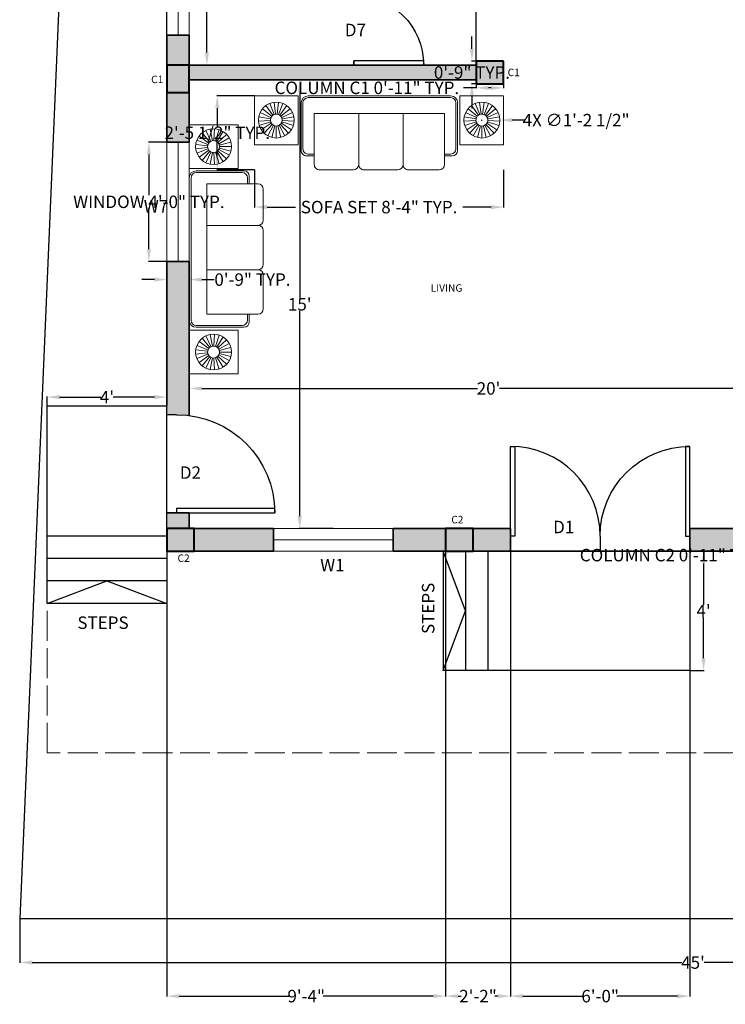
# Model space of a CAD drawing. Units: inches. Extents: x 23868 to 24454, y 31838 to 32477.
# Tile 1 of 4: x 23868 to 24151, y 31838 to 32233. Entities that reach past the tile are written whole.
import ezdxf

# ---------------------------------------------------------------- set-up
doc = ezdxf.new("R2010")
doc.units = ezdxf.units.IN
doc.linetypes.add('ACAD_ISO02W100', pattern=[15, 12, -3])
for name, color, linetype, lineweight in [('A-ANNO-DIMS', 2, 'Continuous', 18), ('A-AREA-IDEN', 7, 'Continuous', 25), ('A-COLS', 7, 'Continuous', 40), ('A-FURN', 30, 'Continuous', 18), ('A-GLAZ', 5, 'Continuous', 18), ('A-WALL', 7, 'Continuous', 35), ('C-PROP', 7, 'Continuous', 25), ('door', 1, 'Continuous', 25), ('steps', 104, 'Continuous', 25), ('text', 7, 'Continuous', 18)]:
    doc.layers.add(name, color=color, linetype=linetype, lineweight=lineweight)
for name, color, linetype, lineweight, true_color in [('A-COLS-PATT', 67, 'Continuous', 13, 0x727430), ('A-FLOR-OVHD', 244, 'ACAD_ISO02W100', 18, 0x991b1e), ('A-WALL-PATT', 250, 'Continuous', 13, 0x413a3c)]:
    doc.layers.add(name, color=color, linetype=linetype, lineweight=lineweight, true_color=true_color)
doc.styles.get("Standard").update_dxf_attribs({"font": 'arial.ttf', "height": 5})
doc.styles.add('style1', font='arial.ttf', dxfattribs={"height": 3})
doc.dimstyles.get("Standard").update_dxf_attribs({"dimtxt": 5, "dimasz": 5, "dimexe": 0.18, "dimexo": 0.0625, "dimgap": 0.09, "dimtad": 0, "dimtih": 1, "dimtoh": 1, "dimzin": 0, "dimdsep": 46, "dimlunit": 3, "dimtxsty": 'Standard', "dimcen": 0.09, "dimadec": 0, "dimazin": 0, "dimtfac": 1, "dimtofl": 0, "dimtmove": 0, "dimatfit": 3, "dimfxl": 1, "dimtolj": 1, "dimtzin": 0, "dimarcsym": 0})

# ---------------------------------------------------------------- blocks, each defined once
blk = doc.blocks.new('*U2')
for p, q in [((0, 0), (0, -100)), ((1000, 0), (1000, -100))]:
    blk.add_line(p, q)
blk.add_lwpolyline([(0, 0), (0, 1000), (43.75, 1000), (43.75, 0)], close=True)
blk.add_arc((0, 0), 1000, 0, 90)
blk = doc.blocks.new('*U6')
for p, q in [((0, 0), (0, -6)), ((36, 0), (36, -6))]:
    blk.add_line(p, q)
blk.add_lwpolyline([(0, 0), (0, 36), (1.75, 36), (1.75, 0)], close=True)
blk.add_arc((0, 0), 36, 0, 90)
blk = doc.blocks.new('*U5')
for p, q in [((0, 0), (0, -6)), ((28, 0), (28, -6))]:
    blk.add_line(p, q)
blk.add_lwpolyline([(0, 0), (0, 28), (1.75, 28), (1.75, 0)], close=True)
blk.add_arc((0, 0), 28, 0, 90)
blk = doc.blocks.new('sofa')
for p, q in [((-58.2, 3.63), (-60.24, 7.96)), ((-57.63, 3.81), (-58.53, 8.51)), ((-57.03, 3.85), (-56.73, 8.63)), ((-56.44, 3.74), (-54.97, 8.29)), ((-59.41, 2.34), (-63.86, 4.1)), ((-59.12, 2.87), (-62.99, 5.68)), ((-58.71, 3.3), (-61.76, 6.99)), ((-55.9, 3.48), (-53.34, 7.52)), ((-55.44, 3.1), (-51.95, 6.38)), ((-55.09, 2.61), (-50.89, 4.92)), ((-59.56, 1.76), (-64.31, 2.36)), ((-59.56, 1.16), (-64.31, 0.56)), ((-59.41, 0.58), (-63.86, -1.18)), ((-59.12, 0.05), (-62.99, -2.76)), ((-55.09, 0.31), (-50.89, -2)), ((-54.87, 2.06), (-50.23, 3.25)), ((-54.87, 0.86), (-50.23, -0.33)), ((-54.79, 1.46), (-50, 1.46)), ((-58.71, -0.38), (-61.76, -4.07)), ((-58.2, -0.71), (-60.24, -5.04)), ((-57.63, -0.89), (-58.53, -5.59)), ((-57.03, -0.93), (-56.73, -5.71)), ((-56.44, -0.82), (-54.97, -5.37)), ((-55.9, -0.56), (-53.34, -4.6)), ((-55.44, -0.18), (-51.95, -3.46)), ((-66.9, -68.18), (-66.9, -11.07)), ((-66.2, -68.18), (-66.2, -11.07)), ((-44.98, -8.25), (-64.08, -8.25)), ((-45.68, -8.96), (-64.08, -8.96)), ((-43.56, -13.5), (-43.56, -11.07)), ((-42.86, -13.5), (-42.86, -10.37)), ((-59.86, -13.5), (-39.37, -13.5)), ((-59.86, -65.75), (-59.86, -13.5)), ((-37.25, -15.62), (-37.25, -28.01)), ((-39.37, -30.13), (-59.86, -30.13)), ((-37.25, -32.25), (-37.25, -45.82)), ((-39.37, -47.94), (-59.86, -47.94)), ((-37.25, -50.06), (-37.25, -63.63)), ((-39.37, -65.75), (-59.86, -65.75)), ((-43.56, -65.75), (-43.56, -68.18)), ((-42.86, -65.75), (-42.86, -68.89)), ((-45.68, -70.3), (-64.08, -70.3)), ((-44.98, -71.01), (-64.08, -71.01)), ((-58.2, -78.8), (-60.24, -74.47)), ((-57.63, -78.62), (-58.53, -73.92)), ((-57.03, -78.58), (-56.73, -73.8)), ((-56.44, -78.69), (-54.97, -74.14)), ((-55.9, -78.95), (-53.34, -74.91)), ((-59.41, -80.09), (-63.86, -78.33)), ((-59.12, -79.56), (-62.99, -76.75)), ((-58.71, -79.12), (-61.76, -75.44)), ((-55.44, -79.33), (-51.95, -76.05)), ((-55.09, -79.82), (-50.89, -77.51)), ((-59.56, -80.67), (-64.31, -80.07)), ((-59.56, -81.27), (-64.31, -81.87)), ((-59.41, -81.85), (-63.86, -83.61)), ((-59.12, -82.38), (-62.99, -85.19)), ((-58.71, -82.81), (-61.76, -86.5)), ((-55.44, -82.61), (-51.95, -85.88)), ((-55.09, -82.12), (-50.89, -84.43)), ((-54.87, -80.37), (-50.23, -79.18)), ((-54.87, -81.56), (-50.23, -82.75)), ((-54.79, -80.97), (-50, -80.97)), ((-58.2, -83.13), (-60.24, -87.47)), ((-57.63, -83.32), (-58.53, -88.02)), ((-57.03, -83.36), (-56.73, -88.14)), ((-56.44, -83.25), (-54.97, -87.8)), ((-55.9, -82.99), (-53.34, -87.03))]:
    blk.add_line(p, q)
for points in [[(-66.96, 10.15), (-47.26, 10.15), (-47.26, -7.32), (-66.96, -7.32)], [(-66.96, -89.66), (-47.26, -89.66), (-47.26, -72.19), (-66.96, -72.19)]]:
    blk.add_lwpolyline(points, close=True)
for centre, radius in [((-57.18, 1.46), 7.18), ((-57.18, 1.46), 2.39), ((-57.18, -80.97), 7.18), ((-57.18, -80.97), 2.39)]:
    blk.add_circle(centre, radius)
for centre, radius, start, end in [((-64.08, -11.07), 2.83, 90, 180), ((-64.08, -11.07), 2.12, 90, 180), ((-45.68, -11.07), 2.12, 0, 90), ((-44.98, -10.37), 2.12, 0, 90), ((-39.37, -15.62), 2.12, 0, 90), ((-39.37, -28.01), 2.12, 270, 0), ((-39.37, -32.25), 2.12, 0, 90), ((-39.37, -45.82), 2.12, 270, 0), ((-39.37, -50.06), 2.12, 0, 90), ((-39.37, -63.63), 2.12, 270, 0), ((-64.08, -68.18), 2.83, 180, 270), ((-64.08, -68.18), 2.12, 180, 270), ((-45.68, -68.18), 2.12, 270, 0), ((-44.98, -68.89), 2.12, 270, 0)]:
    blk.add_arc(centre, radius, start, end)
blk = doc.blocks.new('*D30')
at = {"layer": 'A-ANNO-DIMS', "color": 0, "lineweight": -2, "transparency": 16777216}
for p, q in [((23879.1, 32077.73), (23879.1, 32081.55)), ((23884.1, 32081.37), (23900.61, 32081.37)), ((23922.1, 32081.37), (23905.59, 32081.37)), ((23927.1, 32077.73), (23927.1, 32081.55))]:
    blk.add_line(p, q, dxfattribs=at)
at = {"layer": 'A-ANNO-DIMS', "color": 0, "transparency": 16777216}
for points in [[(23884.1, 32082.2), (23884.1, 32080.54), (23879.1, 32081.37)], [(23922.1, 32082.2), (23922.1, 32080.54), (23927.1, 32081.37)]]:
    blk.add_solid(points, dxfattribs=at)
at = {"layer": 'Defpoints', "color": 0, "transparency": 16777216}
for p in [(23879.1, 32081.37), (23879.1, 32077.66), (23927.1, 32077.66)]:
    blk.add_point(p, dxfattribs=at)
at = {"layer": 'A-ANNO-DIMS', "color": 0, "transparency": 16777216, "insert": (23903.1, 32081.37), "char_height": 5, "attachment_point": 5}
blk.add_mtext("\\A1;4'", dxfattribs=at)
blk = doc.blocks.new('*D33')
at = {"layer": 'A-ANNO-DIMS', "color": 0, "lineweight": -2, "transparency": 16777216}
for p, q in [((23936.1, 32084.78), (23936.1, 32084.66)), ((23941.1, 32084.84), (24051.72, 32084.84)), ((24171.1, 32084.84), (24060.48, 32084.84)), ((24176.1, 32084.9), (24176.1, 32085.02))]:
    blk.add_line(p, q, dxfattribs=at)
at = {"layer": 'A-ANNO-DIMS', "color": 0, "transparency": 16777216}
for points in [[(23941.1, 32085.67), (23941.1, 32084.01), (23936.1, 32084.84)], [(24171.1, 32085.67), (24171.1, 32084.01), (24176.1, 32084.84)]]:
    blk.add_solid(points, dxfattribs=at)
at = {"layer": 'Defpoints', "color": 0, "transparency": 16777216}
for p in [(23936.1, 32084.84), (24176.1, 32084.84), (24176.1, 32084.84)]:
    blk.add_point(p, dxfattribs=at)
at = {"layer": 'A-ANNO-DIMS', "color": 0, "transparency": 16777216, "insert": (24056.1, 32084.84), "char_height": 5, "attachment_point": 5}
blk.add_mtext("\\A1;20'", dxfattribs=at)
blk = doc.blocks.new('*D34')
at = {"layer": 'A-ANNO-DIMS', "color": 0, "lineweight": -2, "transparency": 16777216}
for p, q in [((23993.53, 32208.61), (23980.21, 32208.61)), ((23980.39, 32203.61), (23980.39, 32121.25)), ((23980.39, 32033.61), (23980.39, 32115.97)), ((23993.76, 32028.61), (23980.21, 32028.61))]:
    blk.add_line(p, q, dxfattribs=at)
at = {"layer": 'A-ANNO-DIMS', "color": 0, "transparency": 16777216}
for points in [[(23979.56, 32203.61), (23981.22, 32203.61), (23980.39, 32208.61)], [(23979.56, 32033.61), (23981.22, 32033.61), (23980.39, 32028.61)]]:
    blk.add_solid(points, dxfattribs=at)
at = {"layer": 'Defpoints', "color": 0, "transparency": 16777216}
for p in [(23980.39, 32208.61), (23993.59, 32208.61), (23993.83, 32028.61)]:
    blk.add_point(p, dxfattribs=at)
at = {"layer": 'A-ANNO-DIMS', "color": 0, "transparency": 16777216, "insert": (23980.39, 32118.61), "char_height": 5, "attachment_point": 5}
blk.add_mtext("\\A1;15'", dxfattribs=at)
blk = doc.blocks.new('*D35')
at = {"layer": 'A-ANNO-DIMS', "color": 0, "lineweight": -2, "transparency": 16777216}
for p, q in [((23936.16, 32262.61), (23943.36, 32262.61)), ((23943.18, 32257.61), (23943.18, 32241.2)), ((23943.18, 32219.61), (23943.18, 32236.02)), ((23936.16, 32214.61), (23943.36, 32214.61))]:
    blk.add_line(p, q, dxfattribs=at)
at = {"layer": 'A-ANNO-DIMS', "color": 0, "transparency": 16777216}
for points in [[(23942.35, 32257.61), (23944.01, 32257.61), (23943.18, 32262.61)], [(23942.35, 32219.61), (23944.01, 32219.61), (23943.18, 32214.61)]]:
    blk.add_solid(points, dxfattribs=at)
at = {"layer": 'Defpoints', "color": 0, "transparency": 16777216}
for p in [(23936.1, 32262.61), (23943.18, 32262.61), (23936.1, 32214.61)]:
    blk.add_point(p, dxfattribs=at)
at = {"layer": 'A-ANNO-DIMS', "color": 0, "transparency": 16777216, "insert": (23943.18, 32238.61), "char_height": 5, "attachment_point": 5}
blk.add_mtext("\\A1;4'", dxfattribs=at)
blk = doc.blocks.new('*D39')
at = {"layer": 'A-ANNO-DIMS', "color": 0, "lineweight": -2, "transparency": 16777216}
for p, q in [((24136.92, 32019.61), (24142.52, 32019.61)), ((24142.34, 32014.61), (24142.34, 31998.2)), ((24142.34, 31976.61), (24142.34, 31993.02)), ((24136.92, 31971.61), (24142.52, 31971.61))]:
    blk.add_line(p, q, dxfattribs=at)
at = {"layer": 'A-ANNO-DIMS', "color": 0, "transparency": 16777216}
for points in [[(24141.5, 32014.61), (24143.17, 32014.61), (24142.34, 32019.61)], [(24141.5, 31976.61), (24143.17, 31976.61), (24142.34, 31971.61)]]:
    blk.add_solid(points, dxfattribs=at)
at = {"layer": 'Defpoints', "color": 0, "transparency": 16777216}
for p in [(24136.86, 32019.61), (24142.34, 32019.61), (24136.86, 31971.61)]:
    blk.add_point(p, dxfattribs=at)
at = {"layer": 'A-ANNO-DIMS', "color": 0, "transparency": 16777216, "insert": (24142.34, 31995.61), "char_height": 5, "attachment_point": 5}
blk.add_mtext("\\A1;4'", dxfattribs=at)
blk = doc.blocks.new('*D41')
at = {"layer": 'A-ANNO-DIMS', "color": 0, "lineweight": -2, "transparency": 16777216}
for p, q in [((23868.1, 31871.99), (23868.1, 31854.3)), ((24408.1, 31871.99), (24408.1, 31854.3)), ((23873.1, 31854.48), (24133.67, 31854.48)), ((24403.1, 31854.48), (24142.53, 31854.48))]:
    blk.add_line(p, q, dxfattribs=at)
at = {"layer": 'A-ANNO-DIMS', "color": 0, "transparency": 16777216}
for points in [[(23873.1, 31855.32), (23873.1, 31853.65), (23868.1, 31854.48)], [(24403.1, 31855.32), (24403.1, 31853.65), (24408.1, 31854.48)]]:
    blk.add_solid(points, dxfattribs=at)
at = {"layer": 'Defpoints', "color": 0, "transparency": 16777216}
for p in [(23868.1, 31872.05), (24408.1, 31872.05), (23868.1, 31854.48)]:
    blk.add_point(p, dxfattribs=at)
at = {"layer": 'A-ANNO-DIMS', "color": 0, "transparency": 16777216, "insert": (24138.1, 31854.48), "char_height": 5, "attachment_point": 5}
blk.add_mtext("\\A1;45'", dxfattribs=at)
blk = doc.blocks.new('WIN-48IN')
blk.add_line((0, 4.5), (48, 4.5))
blk.add_lwpolyline([(0, 0), (48, 0), (48, 9), (0, 9)], close=True)
blk = doc.blocks.new('WIN-24IN')
blk.add_line((4.5, 0), (4.5, 24))
blk.add_lwpolyline([(0, 24), (9, 24), (9, 0), (0, 0)], close=True)
blk = doc.blocks.new('COL-C1')
blk.add_lwpolyline([(9, 0), (9, 11.01), (0, 11.01), (0, 0)], close=True)
blk = doc.blocks.new('COL-C2')
blk.add_lwpolyline([(11.01, 9), (0, 9), (0, 0), (11.01, 0)], close=True)
blk = doc.blocks.new('*D47')
at = {"layer": 'A-ANNO-DIMS', "color": 0, "lineweight": -2, "transparency": 16777216}
for p, q in [((24051.09, 32205.46), (24046.09, 32205.46)), ((24051.09, 32207.05), (24051.09, 32205.28)), ((24057.1, 32205.46), (24056.09, 32205.46)), ((24062.1, 32207.05), (24062.1, 32205.28))]:
    blk.add_line(p, q, dxfattribs=at)
at = {"layer": 'A-ANNO-DIMS', "color": 0, "transparency": 16777216}
for points in [[(24056.09, 32206.29), (24056.09, 32204.62), (24051.09, 32205.46)], [(24057.1, 32206.29), (24057.1, 32204.62), (24062.1, 32205.46)]]:
    blk.add_solid(points, dxfattribs=at)
at = {"layer": 'Defpoints', "color": 0, "transparency": 16777216}
for p in [(24051.09, 32207.11), (24051.09, 32205.46), (24062.1, 32207.11)]:
    blk.add_point(p, dxfattribs=at)
at = {"layer": 'A-ANNO-DIMS', "color": 0, "transparency": 16777216, "insert": (24007.31, 32205.46), "char_height": 5, "attachment_point": 5}
blk.add_mtext('\\A1;COLUMN C1 0\'-11" TYP.', dxfattribs=at)
blk = doc.blocks.new('*D48')
at = {"layer": 'A-ANNO-DIMS', "color": 0, "lineweight": -2, "transparency": 16777216}
for p, q in [((24049.44, 32221.11), (24049.44, 32226.11)), ((24051.03, 32216.11), (24049.26, 32216.11)), ((24051.03, 32207.11), (24049.26, 32207.11)), ((24049.44, 32202.11), (24049.44, 32197.11))]:
    blk.add_line(p, q, dxfattribs=at)
at = {"layer": 'A-ANNO-DIMS', "color": 0, "transparency": 16777216}
for points in [[(24048.6, 32221.11), (24050.27, 32221.11), (24049.44, 32216.11)], [(24048.6, 32202.11), (24050.27, 32202.11), (24049.44, 32207.11)]]:
    blk.add_solid(points, dxfattribs=at)
at = {"layer": 'Defpoints', "color": 0, "transparency": 16777216}
for p in [(24049.44, 32216.11), (24051.09, 32216.11), (24051.09, 32207.11)]:
    blk.add_point(p, dxfattribs=at)
at = {"layer": 'A-ANNO-DIMS', "color": 0, "transparency": 16777216, "insert": (24049.44, 32211.61), "char_height": 5, "attachment_point": 5}
blk.add_mtext('\\A1;0\'-9" TYP.', dxfattribs=at)
blk = doc.blocks.new('*D49')
at = {"layer": 'A-ANNO-DIMS', "color": 0, "lineweight": -2, "transparency": 16777216}
for p, q in [((24173.47, 32017.96), (24168.47, 32017.96)), ((24173.47, 32019.55), (24173.47, 32017.78)), ((24179.48, 32017.96), (24178.47, 32017.96)), ((24184.48, 32019.55), (24184.48, 32017.78))]:
    blk.add_line(p, q, dxfattribs=at)
at = {"layer": 'A-ANNO-DIMS', "color": 0, "transparency": 16777216}
for points in [[(24178.47, 32018.79), (24178.47, 32017.12), (24173.47, 32017.96)], [(24179.48, 32018.79), (24179.48, 32017.12), (24184.48, 32017.96)]]:
    blk.add_solid(points, dxfattribs=at)
at = {"layer": 'Defpoints', "color": 0, "transparency": 16777216}
for p in [(24173.47, 32019.61), (24173.47, 32017.96), (24184.48, 32019.61)]:
    blk.add_point(p, dxfattribs=at)
at = {"layer": 'A-ANNO-DIMS', "color": 0, "transparency": 16777216, "insert": (24129.69, 32017.96), "char_height": 5, "attachment_point": 5}
blk.add_mtext('\\A1;COLUMN C2 0\'-11" TYP.', dxfattribs=at)
blk = doc.blocks.new('*D51')
at = {"layer": 'A-ANNO-DIMS', "color": 0, "lineweight": -2, "transparency": 16777216}
for p, q in [((23927.04, 32183.72), (23919.72, 32183.72)), ((23919.9, 32178.72), (23919.9, 32162.4)), ((23919.9, 32140.72), (23919.9, 32157.04)), ((23927.04, 32135.72), (23919.72, 32135.72))]:
    blk.add_line(p, q, dxfattribs=at)
at = {"layer": 'A-ANNO-DIMS', "color": 0, "transparency": 16777216}
for points in [[(23919.07, 32178.72), (23920.73, 32178.72), (23919.9, 32183.72)], [(23919.07, 32140.72), (23920.73, 32140.72), (23919.9, 32135.72)]]:
    blk.add_solid(points, dxfattribs=at)
at = {"layer": 'Defpoints', "color": 0, "transparency": 16777216}
for p in [(23927.1, 32183.72), (23919.9, 32135.72), (23927.1, 32135.72)]:
    blk.add_point(p, dxfattribs=at)
at = {"layer": 'A-ANNO-DIMS', "color": 0, "transparency": 16777216, "insert": (23919.9, 32159.72), "char_height": 5, "attachment_point": 5}
blk.add_mtext('\\A1;WINDOW 4\'-0" TYP.', dxfattribs=at)
blk = doc.blocks.new('*D52')
at = {"layer": 'A-ANNO-DIMS', "color": 0, "lineweight": -2, "transparency": 16777216}
for p, q in [((23927.1, 32135.66), (23927.1, 32128.34)), ((23936.1, 32135.66), (23936.1, 32128.34)), ((23922.1, 32128.52), (23917.1, 32128.52)), ((23941.1, 32128.52), (23946.1, 32128.52))]:
    blk.add_line(p, q, dxfattribs=at)
at = {"layer": 'A-ANNO-DIMS', "color": 0, "transparency": 16777216}
for points in [[(23922.1, 32129.35), (23922.1, 32127.69), (23927.1, 32128.52)], [(23941.1, 32129.35), (23941.1, 32127.69), (23936.1, 32128.52)]]:
    blk.add_solid(points, dxfattribs=at)
at = {"layer": 'Defpoints', "color": 0, "transparency": 16777216}
for p in [(23927.1, 32135.72), (23936.1, 32135.72), (23936.1, 32128.52)]:
    blk.add_point(p, dxfattribs=at)
at = {"layer": 'A-ANNO-DIMS', "color": 0, "transparency": 16777216, "insert": (23961.43, 32128.52), "char_height": 5, "attachment_point": 5}
blk.add_mtext('\\A1;0\'-9" TYP.', dxfattribs=at)
blk = doc.blocks.new('*D57')
at = {"layer": 'A-ANNO-DIMS', "color": 0, "lineweight": -2, "transparency": 16777216}
for p, q in [((23962.31, 32172.51), (23962.31, 32157.42)), ((24062.12, 32172.51), (24062.12, 32157.42)), ((23967.31, 32157.6), (23978.65, 32157.6)), ((24057.12, 32157.6), (24045.77, 32157.6))]:
    blk.add_line(p, q, dxfattribs=at)
at = {"layer": 'A-ANNO-DIMS', "color": 0, "transparency": 16777216}
for points in [[(23967.31, 32158.43), (23967.31, 32156.77), (23962.31, 32157.6)], [(24057.12, 32158.43), (24057.12, 32156.77), (24062.12, 32157.6)]]:
    blk.add_solid(points, dxfattribs=at)
at = {"layer": 'Defpoints', "color": 0, "transparency": 16777216}
for p in [(23962.31, 32172.57), (24062.12, 32172.57), (24062.12, 32157.6)]:
    blk.add_point(p, dxfattribs=at)
at = {"layer": 'A-ANNO-DIMS', "color": 0, "transparency": 16777216, "insert": (24012.21, 32157.6), "char_height": 5, "attachment_point": 5}
blk.add_mtext('\\A1;SOFA SET 8\'-4" TYP.', dxfattribs=at)
blk = doc.blocks.new('*D58')
at = {"layer": 'A-ANNO-DIMS', "color": 0, "lineweight": -2, "transparency": 16777216}
for p, q in [((23962.24, 32202.29), (23947.15, 32202.29)), ((23947.33, 32197.29), (23947.33, 32190.11)), ((23947.33, 32177.57), (23947.33, 32184.76)), ((23962.24, 32172.57), (23947.15, 32172.57))]:
    blk.add_line(p, q, dxfattribs=at)
at = {"layer": 'A-ANNO-DIMS', "color": 0, "transparency": 16777216}
for points in [[(23946.5, 32197.29), (23948.17, 32197.29), (23947.33, 32202.29)], [(23946.5, 32177.57), (23948.17, 32177.57), (23947.33, 32172.57)]]:
    blk.add_solid(points, dxfattribs=at)
at = {"layer": 'Defpoints', "color": 0, "transparency": 16777216}
for p in [(23962.31, 32202.29), (23947.33, 32172.57), (23962.31, 32172.57)]:
    blk.add_point(p, dxfattribs=at)
at = {"layer": 'A-ANNO-DIMS', "color": 0, "transparency": 16777216, "insert": (23947.33, 32187.43), "char_height": 5, "attachment_point": 5}
blk.add_mtext('\\A1;2\'-5 1/2" TYP.', dxfattribs=at)
blk = doc.blocks.new('*D69')
at = {"layer": 'A-ANNO-DIMS', "color": 0, "lineweight": -2, "transparency": 16777216}
for p, q in [((23927.1, 32019.55), (23927.1, 31840.82)), ((24038.91, 32019.55), (24038.91, 31840.82)), ((23932.1, 31841), (23976.27, 31841)), ((24033.91, 31841), (23989.74, 31841))]:
    blk.add_line(p, q, dxfattribs=at)
at = {"layer": 'A-ANNO-DIMS', "color": 0, "transparency": 16777216}
for points in [[(23932.1, 31841.83), (23932.1, 31840.17), (23927.1, 31841)], [(24033.91, 31841.83), (24033.91, 31840.17), (24038.91, 31841)]]:
    blk.add_solid(points, dxfattribs=at)
at = {"layer": 'Defpoints', "color": 0, "transparency": 16777216}
for p in [(23927.1, 32019.61), (24038.91, 32019.61), (24038.91, 31841)]:
    blk.add_point(p, dxfattribs=at)
at = {"layer": 'A-ANNO-DIMS', "color": 0, "transparency": 16777216, "insert": (23983, 31841), "char_height": 5, "attachment_point": 5}
blk.add_mtext('\\A1;9\'-4"', dxfattribs=at)
blk = doc.blocks.new('*D70')
at = {"layer": 'A-ANNO-DIMS', "color": 0, "lineweight": -2, "transparency": 16777216}
for p, q in [((23927.1, 32214.67), (23927.1, 32473.68)), ((23932.1, 32473.5), (23980.65, 32473.5)), ((24046.09, 32473.5), (23997.54, 32473.5)), ((24051.09, 32216.17), (24051.09, 32473.68))]:
    blk.add_line(p, q, dxfattribs=at)
at = {"layer": 'A-ANNO-DIMS', "color": 0, "transparency": 16777216}
for points in [[(23932.1, 32474.34), (23932.1, 32472.67), (23927.1, 32473.5)], [(24046.09, 32474.34), (24046.09, 32472.67), (24051.09, 32473.5)]]:
    blk.add_solid(points, dxfattribs=at)
at = {"layer": 'Defpoints', "color": 0, "transparency": 16777216}
for p in [(24051.09, 32473.5), (24051.09, 32216.11), (23927.1, 32214.61)]:
    blk.add_point(p, dxfattribs=at)
at = {"layer": 'A-ANNO-DIMS', "color": 0, "transparency": 16777216, "insert": (23989.09, 32473.5), "char_height": 5, "attachment_point": 5}
blk.add_mtext('\\A1;10\'-4"', dxfattribs=at)
blk = doc.blocks.new('*D71')
at = {"layer": 'A-ANNO-DIMS', "color": 0, "lineweight": -2, "transparency": 16777216}
for p, q in [((24038.91, 32019.55), (24038.91, 31840.82)), ((24064.86, 32019.55), (24064.86, 31840.82)), ((24043.91, 31841), (24045.11, 31841)), ((24059.86, 31841), (24058.66, 31841))]:
    blk.add_line(p, q, dxfattribs=at)
at = {"layer": 'A-ANNO-DIMS', "color": 0, "transparency": 16777216}
for points in [[(24043.91, 31841.83), (24043.91, 31840.17), (24038.91, 31841)], [(24059.86, 31841.83), (24059.86, 31840.17), (24064.86, 31841)]]:
    blk.add_solid(points, dxfattribs=at)
at = {"layer": 'Defpoints', "color": 0, "transparency": 16777216}
for p in [(24038.91, 32019.61), (24064.86, 32019.61), (24064.86, 31841)]:
    blk.add_point(p, dxfattribs=at)
at = {"layer": 'A-ANNO-DIMS', "color": 0, "transparency": 16777216, "insert": (24051.88, 31841), "char_height": 5, "attachment_point": 5}
blk.add_mtext('\\A1;2\'-2"', dxfattribs=at)
blk = doc.blocks.new('*D72')
at = {"layer": 'A-ANNO-DIMS', "color": 0, "lineweight": -2, "transparency": 16777216}
for p, q in [((24064.86, 32019.55), (24064.86, 31840.82)), ((24136.86, 32019.55), (24136.86, 31840.82)), ((24069.86, 31841), (24094.11, 31841)), ((24131.86, 31841), (24107.61, 31841))]:
    blk.add_line(p, q, dxfattribs=at)
at = {"layer": 'A-ANNO-DIMS', "color": 0, "transparency": 16777216}
for points in [[(24069.86, 31841.83), (24069.86, 31840.17), (24064.86, 31841)], [(24131.86, 31841.83), (24131.86, 31840.17), (24136.86, 31841)]]:
    blk.add_solid(points, dxfattribs=at)
at = {"layer": 'Defpoints', "color": 0, "transparency": 16777216}
for p in [(24064.86, 32019.61), (24136.86, 32019.61), (24136.86, 31841)]:
    blk.add_point(p, dxfattribs=at)
at = {"layer": 'A-ANNO-DIMS', "color": 0, "transparency": 16777216, "insert": (24100.86, 31841), "char_height": 5, "attachment_point": 5}
blk.add_mtext('\\A1;6\'-0"', dxfattribs=at)
blk = doc.blocks.new('*D74')
at = {"layer": 'A-ANNO-DIMS', "color": 0, "lineweight": -2, "transparency": 16777216}
for p, q in [((24053.34, 32192.51), (24053.52, 32192.51)), ((24053.43, 32192.42), (24053.43, 32192.6)), ((24070.61, 32192.51), (24065.61, 32192.51))]:
    blk.add_line(p, q, dxfattribs=at)
at = {"layer": 'A-ANNO-DIMS', "color": 0, "transparency": 16777216}
blk.add_solid([(24065.61, 32193.34), (24065.61, 32191.68), (24060.61, 32192.51)], dxfattribs=at)
at = {"layer": 'Defpoints', "color": 0, "transparency": 16777216}
for p in [(24046.25, 32192.51), (24060.61, 32192.51)]:
    blk.add_point(p, dxfattribs=at)
at = {"layer": 'A-ANNO-DIMS', "color": 0, "transparency": 16777216, "insert": (24091.23, 32192.51), "char_height": 5, "attachment_point": 5}
blk.add_mtext('\\A1;4X ∅1\'-2 1/2"', dxfattribs=at)

msp = doc.modelspace()

# ---------------------------------------------------------------- hatches: boundary and pattern name
at = {"layer": 'A-COLS-PATT'}
h = msp.add_hatch(color=256, dxfattribs=at)
h.dxf.hatch_style = 1
h.paths.add_polyline_path([(23938.111, 32028.608), (23927.1, 32028.608), (23927.1, 32019.608), (23938.111, 32019.608)])
h.paths.add_polyline_path([(24049.921, 32028.608), (24038.91, 32028.608), (24038.91, 32019.608), (24049.921, 32019.608)])
h.paths.add_polyline_path([(24184.484, 32028.608), (24173.473, 32028.608), (24173.473, 32019.608), (24184.484, 32019.608)])
h.paths.add_polyline_path([(24371.1, 32028.608), (24360.089, 32028.608), (24360.089, 32019.608), (24371.1, 32019.608)])
h.paths.add_polyline_path([(24371.1, 32214.608), (24362.1, 32214.608), (24362.1, 32203.597), (24371.1, 32203.597)])
h.paths.add_polyline_path([(24185.1, 32214.608), (24176.1, 32214.608), (24176.1, 32203.597), (24185.1, 32203.597)])
h.paths.add_polyline_path([(24062.1, 32216.108), (24051.089, 32216.108), (24051.089, 32207.108), (24062.1, 32207.108)])
h.paths.add_polyline_path([(24371.1, 32403.608), (24360.089, 32403.608), (24360.089, 32394.608), (24371.1, 32394.608)])
h.paths.add_polyline_path([(24187.111, 32403.608), (24176.1, 32403.608), (24176.1, 32394.608), (24187.111, 32394.608)])
h.paths.add_polyline_path([(24065.1, 32403.608), (24056.1, 32403.608), (24056.1, 32392.597), (24065.1, 32392.597)])
h.paths.add_polyline_path([(23936.1, 32403.608), (23927.1, 32403.608), (23927.1, 32392.597), (23936.1, 32392.597)])
h.paths.add_polyline_path([(23936.1, 32214.608), (23927.1, 32214.608), (23927.1, 32203.597), (23936.1, 32203.597)])
at = {"layer": 'A-WALL-PATT'}
h = msp.add_hatch(color=256, dxfattribs=at)
h.dxf.hatch_style = 1
h.paths.add_polyline_path([(23927.1, 32203.597), (23927.1, 32183.719), (23936.043, 32183.719), (23936.043, 32190.568), (23936.074, 32203.597)])
h.paths.add_polyline_path([(23936.1, 32226.608), (23927.1, 32226.608), (23927.1, 32214.608), (23936.1, 32214.608)])
h.paths.add_polyline_path([(24051.089, 32214.608), (23936.1, 32214.608), (23936.1, 32208.608), (24051.089, 32208.608)])
h = msp.add_hatch(color=256, dxfattribs=at)
h.dxf.hatch_style = 1
h.paths.add_polyline_path([(23969.827, 32028.608), (23938.111, 32028.608), (23938.111, 32019.608), (23969.827, 32019.608)])
h.paths.add_polyline_path([(23936.1, 32034.899), (23931.037, 32034.899), (23927.1, 32034.899), (23927.1, 32028.608), (23936.1, 32028.608)])
h.paths.add_polyline_path([(24038.91, 32028.608), (24017.827, 32028.608), (24017.827, 32019.608), (24038.91, 32019.608)])
h.paths.add_polyline_path([(24064.858, 32028.608), (24049.921, 32028.608), (24049.921, 32019.608), (24064.858, 32019.608)])
h.paths.add_polyline_path([(24173.473, 32028.608), (24136.858, 32028.608), (24136.858, 32025.608), (24136.858, 32019.608), (24173.473, 32019.608)])
h.paths.add_polyline_path([(24221.1, 32028.608), (24184.484, 32028.608), (24184.484, 32019.608), (24221.1, 32019.608)])
h.paths.add_polyline_path([(24360.089, 32028.608), (24269.1, 32028.608), (24269.1, 32019.608), (24360.089, 32019.608)])
h.paths.add_polyline_path([(24314.1, 32079.817), (24308.1, 32079.817), (24308.1, 32028.608), (24314.1, 32028.608)])
h.paths.add_polyline_path([(24371.1, 32060.108), (24362.1, 32060.108), (24362.1, 32028.608), (24371.1, 32028.608)])
h.paths.add_polyline_path([(24371.1, 32150.603), (24362.1, 32150.603), (24362.1, 32084.108), (24371.1, 32084.108)])
h.paths.add_polyline_path([(24362.1, 32121.608), (24314.1, 32121.608), (24314.1, 32208.608), (24318.636, 32208.608), (24318.636, 32214.608), (24185.1, 32214.608), (24185.1, 32208.608), (24308.1, 32208.608), (24308.1, 32107.817), (24314.1, 32107.817), (24314.1, 32115.608), (24362.1, 32115.608)])
h.paths.add_polyline_path([(24371.1, 32203.597), (24362.1, 32203.597), (24362.1, 32174.603), (24371.1, 32174.603)])
h = msp.add_hatch(color=256, dxfattribs=at)
h.dxf.hatch_style = 1
h.paths.add_polyline_path([(23936.1, 32135.719), (23927.1, 32135.719), (23927.1, 32077.664), (23927.1, 32074.269), (23931.037, 32074.269, -0.0322505), (23936.1, 32073.942), (23936.1, 32090.753), (23936.043, 32090.753), (23936.043, 32108.225)])

# ---------------------------------------------------------------- linework, layer by layer
at = {"layer": 'A-FLOR-OVHD'}
for p, q in [((23879.1, 31938.608), (23879.1, 31998.608)), ((24214.383, 31938.608), (23879.1, 31938.608))]:
    msp.add_line(p, q, dxfattribs=at)
at = {"layer": 'A-WALL'}
for p, q in [((23936.1, 32226.608), (23927.1, 32226.608)), ((23936.1, 32214.608), (23936.1, 32226.608)), ((24002.1, 32214.608), (24002.1, 32216.358)), ((23936.1, 32214.608), (24051.089, 32214.608)), ((23936.1, 32183.719), (23936.1, 32214.608)), ((24062.1, 32208.608), (24062.1, 32214.608)), ((23936.1, 32208.608), (24051.089, 32208.608)), ((23927.1, 32183.719), (23936.1, 32183.719)), ((23927.1, 32135.719), (23936.1, 32135.719)), ((23936.1, 32073.942), (23936.1, 32135.719)), ((23936.1, 32034.899), (23927.1, 32034.899)), ((23936.1, 32028.608), (23936.1, 32034.899)), ((23969.827, 32028.608), (23936.1, 32028.608)), ((23969.827, 32019.608), (23969.827, 32028.608)), ((24017.827, 32019.608), (24017.827, 32028.608)), ((24064.858, 32028.608), (24017.827, 32028.608)), ((24064.858, 32019.608), (24064.858, 32028.608)), ((24100.983, 32028.608), (24100.733, 32028.608)), ((24136.858, 32019.608), (24136.858, 32028.608)), ((24221.1, 32028.608), (24136.858, 32028.608)), ((24064.858, 32019.608), (24136.858, 32019.608))]:
    msp.add_line(p, q, dxfattribs=at)
for points in [[(23927.1, 32183.719), (23927.1, 32226.608)], [(23927.1, 32077.664), (23927.1, 32135.719)], [(23969.827, 32019.608), (23927.1, 32019.608)], [(24064.858, 32019.608), (24017.827, 32019.608)], [(24221.1, 32019.608), (24136.858, 32019.608)]]:
    msp.add_lwpolyline(points, dxfattribs=at)
at = {"layer": 'C-PROP'}
for p in [(23892.456, 32442.452), (23892.136, 32434.947), (24408.1, 31872.048)]:
    msp.add_line(p, (23868.1, 31872.048), dxfattribs=at)
at = {"layer": 'steps'}
for p, q in [((23927.1, 32077.664), (23879.1, 32077.664)), ((23927.1, 32025.608), (23879.1, 32025.608)), ((23927.1, 32019.608), (23927.1, 31998.608)), ((24037.858, 32019.608), (24037.858, 31971.608)), ((24046.858, 31995.608), (24037.858, 32019.608)), ((24046.858, 32019.608), (24046.858, 31971.608)), ((24055.858, 32019.608), (24055.858, 31971.608)), ((24064.858, 32019.608), (24064.858, 31971.608)), ((24136.858, 32019.608), (24136.858, 31971.608)), ((23927.1, 32016.608), (23879.1, 32016.608)), ((23927.1, 32007.608), (23879.1, 32007.608)), ((23879.1, 31998.608), (23903.1, 32007.608)), ((23903.1, 32007.608), (23927.1, 31998.608)), ((23927.1, 31998.608), (23879.1, 31998.608)), ((24037.858, 31971.608), (24046.858, 31995.608)), ((24064.858, 31971.608), (24037.858, 31971.608)), ((24136.858, 31971.608), (24064.858, 31971.608))]:
    msp.add_line(p, q, dxfattribs=at)
for points in [[(23879.1, 31998.608), (23879.1, 32077.664)], [(23927.1, 32019.608), (23927.1, 32077.664)]]:
    msp.add_lwpolyline(points, dxfattribs=at)

# ---------------------------------------------------------------- block references
at = {"layer": 'A-COLS', "rotation": 90.00000000001894}
msp.add_blockref('COL-C1', (24062.1, 32207.108), dxfattribs=at)
at = {"layer": 'A-COLS'}
for name, p in [('COL-C1', (23927.1, 32203.597)), ('COL-C2', (23927.1, 32019.608)), ('COL-C2', (24038.91, 32019.608))]:
    msp.add_blockref(name, p, dxfattribs=at)
at = {"layer": 'A-FURN', "rotation": 270}
msp.add_blockref('sofa', (24051.968, 32135.327), dxfattribs=at)
at = {"layer": 'A-FURN'}
msp.add_blockref('sofa', (24003.004, 32180.415), dxfattribs=at)
at = {"layer": 'A-GLAZ'}
for name, p in [('WIN-24IN', (23927.1, 32226.608)), ('WIN-48IN', (23969.827, 32019.608))]:
    msp.add_blockref(name, p, dxfattribs=at)
at = {"layer": 'A-GLAZ', "rotation": 270}
msp.add_blockref('WIN-48IN', (23927.1, 32183.72), dxfattribs=at)
at = {"layer": 'door', "xscale": -1, "rotation": 270}
msp.add_blockref('*U5', (24002.1, 32214.608), dxfattribs=at)
at = {"layer": 'door', "xscale": -0.0393700787401575, "yscale": 0.0393700787401575, "zscale": 0.0393700787401575, "rotation": 270}
msp.add_blockref('*U2', (23931.037, 32034.899), dxfattribs=at)
at = {"layer": 'door'}
msp.add_blockref('*U6', (24064.858, 32025.608), dxfattribs=at)
at = {"layer": 'door', "xscale": -1}
msp.add_blockref('*U6', (24136.858, 32025.608), dxfattribs=at)

# ---------------------------------------------------------------- texts
at = {"layer": 'A-AREA-IDEN', "insert": (24032.877, 32126.644), "char_height": 3, "attachment_point": 1, "style": 'style1'}
msp.add_mtext_dynamic_manual_height_columns('LIVING', width=43.29926, gutter_width=15, heights=[0], dxfattribs=at)
at = {"layer": 'text', "char_height": 5, "attachment_point": 1}
for s, width, gutter_width, insert in [('D7', 9.30203, 12.5, (23998.475, 32231.168)), ('W7', 9.30203, 12.5, (23917.859, 32160.4)), ('D2', 9.30203, 12.5, (23932.32, 32053.574)), ('D1', 9.4115, 25, (24082.011, 32031.739)), ('W1', 9.30203, 12.5, (23988.597, 32016.452)), ('STEPS', 25.97022, 25, (23891.231, 31993.34))]:
    msp.add_mtext_dynamic_manual_height_columns(s, width=width, gutter_width=gutter_width, heights=[0], dxfattribs=dict(at, insert=insert))
at = {"layer": 'text', "char_height": 3, "attachment_point": 1, "style": 'style1'}
for s, insert in [('C1', (24063.77, 32213.141)), ('C1', (23920.798, 32210.348)), ('C2', (24041.154, 32033.708)), ('C2', (23931.391, 32018.228))]:
    msp.add_mtext_dynamic_manual_height_columns(s, width=6.09517, gutter_width=15, heights=[0], dxfattribs=dict(at, insert=insert))
at = {"layer": 'text', "insert": (24029.389, 31986.314), "char_height": 5, "attachment_point": 1, "rotation": 90}
msp.add_mtext_dynamic_manual_height_columns('STEPS', width=17.96695, gutter_width=25, heights=[0], dxfattribs=at)

# ---------------------------------------------------------------- dimensions: what is measured, and where the dimension line sits
at = {"layer": 'A-ANNO-DIMS'}
for base, p1, p2, override, picture, middle in [((24051.089, 32473.503), (23927.1, 32214.608), (24051.089, 32216.108), {"dimdec": 1, "dimlfac": 1, "dimrnd": 0, "dimzin": 1, "dimdsep": 46, "dimlunit": 4, "dimfrac": 2}, '*D70', (23989.094, 32473.503)), ((24176.1, 32084.84), (23936.1, 32084.84), (24176.1, 32084.84), {"dimclrd": 0, "dimclre": 0, "dimclrt": 0}, '*D33', (24056.1, 32084.84)), ((23879.1, 32081.371), (23927.1, 32077.664), (23879.1, 32077.664), {"dimclrd": 0, "dimclre": 0, "dimclrt": 0}, '*D30', (23903.1, 32081.371)), ((24038.91, 31840.998), (23927.1, 32019.608), (24038.91, 32019.608), {"dimdec": 1, "dimlfac": 1, "dimrnd": 0, "dimzin": 1, "dimdsep": 46, "dimlunit": 4, "dimfrac": 2}, '*D69', (23983.005, 31840.998)), ((24064.858, 31840.998), (24038.91, 32019.608), (24064.858, 32019.608), {"dimdec": 1, "dimlfac": 1, "dimrnd": 0, "dimzin": 1, "dimdsep": 46, "dimlunit": 4, "dimfrac": 2}, '*D71', (24051.884, 31840.998)), ((24136.858, 31840.998), (24064.858, 32019.608), (24136.858, 32019.608), {"dimdec": 1, "dimlfac": 1, "dimrnd": 0, "dimzin": 1, "dimdsep": 46, "dimlunit": 4, "dimfrac": 2}, '*D72', (24100.858, 31840.998)), ((23868.1, 31854.482), (24408.1, 31872.048), (23868.1, 31872.048), {"dimclrd": 0, "dimclre": 0, "dimclrt": 0}, '*D41', (24138.1, 31854.482))]:
    dim = msp.add_linear_dim(base=base, p1=p1, p2=p2, dimstyle='Standard', override=override, dxfattribs=at)
    dim.commit()
    dim.dimension.update_dxf_attribs({"geometry": picture, "text_midpoint": middle})
for base, p1, p2, picture, middle in [((23943.178, 32262.608), (23936.1, 32214.608), (23936.1, 32262.608), '*D35', (23943.178, 32238.608)), ((23980.391, 32208.608), (23993.827, 32028.608), (23993.594, 32208.608), '*D34', (23980.391, 32118.608)), ((24142.336, 32019.608), (24136.858, 31971.608), (24136.858, 32019.608), '*D39', (24142.336, 31995.608))]:
    dim = msp.add_linear_dim(base=base, p1=p1, p2=p2, angle=90, dimstyle='Standard', override={"dimclrd": 0, "dimclre": 0, "dimclrt": 0}, dxfattribs=at)
    dim.commit()
    dim.dimension.update_dxf_attribs({"geometry": picture, "text_midpoint": middle})
for base, p1, p2, angle, text, picture, middle in [((24049.437, 32216.108), (24051.089, 32207.108), (24051.089, 32216.108), 90, '<> TYP.', '*D48', (24049.437, 32211.608)), ((24051.089, 32205.457), (24062.1, 32207.108), (24051.089, 32207.108), 180, 'COLUMN C1 <> TYP.', '*D47', (24007.307, 32205.457)), ((23947.334, 32172.574), (23962.306, 32202.287), (23962.306, 32172.574), 270, '<> TYP.', '*D58', (23947.334, 32187.431)), ((23919.9, 32135.719), (23927.1, 32183.719), (23927.1, 32135.719), 270, 'WINDOW <> TYP.', '*D51', (23919.9, 32159.719)), ((24173.473, 32017.957), (24184.484, 32019.608), (24173.473, 32019.608), 180, 'COLUMN C2 <> TYP.', '*D49', (24129.691, 32017.957))]:
    dim = msp.add_linear_dim(base=base, p1=p1, p2=p2, angle=angle, text=text, dimstyle='Standard', override={"dimdec": 1, "dimlfac": 1, "dimrnd": 0, "dimzin": 1, "dimdsep": 46, "dimlunit": 4, "dimfrac": 2}, dxfattribs=at)
    dim.commit()
    dim.dimension.update_dxf_attribs({"geometry": picture, "text_midpoint": middle})
dim = msp.add_diameter_dim_2p(p1=(24046.247, 32192.511), p2=(24060.609, 32192.511), text='4X <>', dimstyle='Standard', override={"dimdec": 1, "dimlfac": 1, "dimrnd": 0, "dimzin": 1, "dimdsep": 46, "dimlunit": 4, "dimfrac": 2}, dxfattribs=at)
dim.commit()
dim.dimension.update_dxf_attribs({"geometry": '*D74', "text_midpoint": (24070.609, 32192.511), "dimtype": 163})
for base, p1, p2, text, picture, middle in [((24062.12, 32157.601), (23962.306, 32172.574), (24062.12, 32172.574), 'SOFA SET <> TYP.', '*D57', (24012.213, 32157.601)), ((23936.1, 32128.519), (23927.1, 32135.719), (23936.1, 32135.719), '<> TYP.', '*D52', (23961.429, 32128.519))]:
    dim = msp.add_linear_dim(base=base, p1=p1, p2=p2, text=text, dimstyle='Standard', override={"dimdec": 1, "dimlfac": 1, "dimrnd": 0, "dimzin": 1, "dimdsep": 46, "dimlunit": 4, "dimfrac": 2}, dxfattribs=at)
    dim.commit()
    dim.dimension.update_dxf_attribs({"geometry": picture, "text_midpoint": middle})

doc.saveas('drawing.dxf')
